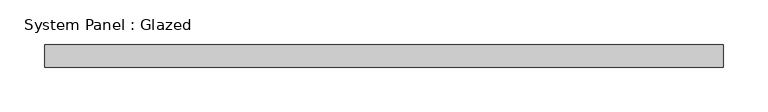
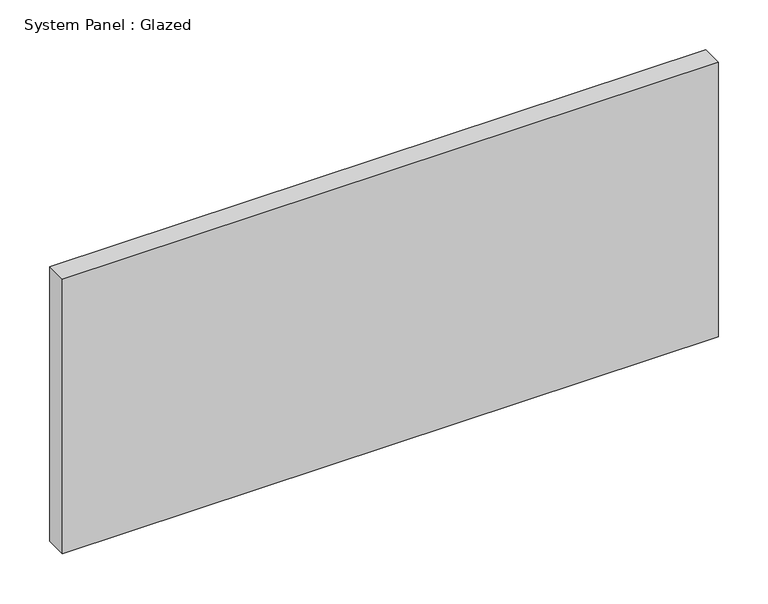
"""IFC4 building model written with IfcOpenShell, lengths in millimetres: plate geometry, System Panel : Glazed."""

from ifc_helpers import new_model, si_unit, origin, origin_with_axes, place, context, project, spatial, polyline, outline, extrude, source, transform, mapped, element, save


def system_panel_glazed_4f752865(model_context):
    return source(origin(), model_context, "Body", "SweptSolid", [
        extrude(outline(polyline([(381.0, 19.05), (-381.0, 19.05), (-381.0, 44.45), (381.0, 44.45), (381.0, 19.05)])), origin_with_axes(), (0.0, 0.0, 1.0), 337.0177198),
    ])


if __name__ == "__main__":
    model = new_model("IFC4")
    model_context = context("Model", 3, world=origin())
    ifc_project = project(units=[si_unit("LENGTHUNIT", "METRE", prefix="MILLI")], contexts=[model_context])
    site = spatial("IfcSite", under=ifc_project)
    building = spatial("IfcBuilding", under=site)
    placement = place(None, origin())
    system_panel_glazed_shape = system_panel_glazed_4f752865(model_context)
    element("IfcPlate", 1, ObjectType="System Panel : Glazed", at=placement, inside=building, context=model_context, shape_type="MappedRepresentation", body=[
        mapped(system_panel_glazed_shape, transform((0.0, 0.0, 0.0), x_axis=(1.0, 0.0, 0.0), y_axis=(0.0, 1.0, 0.0), z_axis=(0.0, 0.0, 1.0))),
    ])
    save(model, "model.ifc")

# Revit data of these elements
# Type "System Panel : Glazed"
#   Construction Type Id = "GSP4R"
#   Analytic Construction = "1/8 in Pilkington single glazing"
#   Visual Light Transmittance = 0.9
#   Solar Heat Gain Coefficient = 0.86
#   Heat Transfer Coefficient (U) = 1.18115 BTU/(h·ft²·°F)
#   Define Thermal Properties by = 1
# Element 1 (IfcPlate, "System Panel : Glazed")
#   Materials on its faces: "Glass"
# Materials
#   "Glass": class "Glass", colour RGB 0 128 192, transparency 0.75, Description = "Soda Lime Glass", Cost = 0
